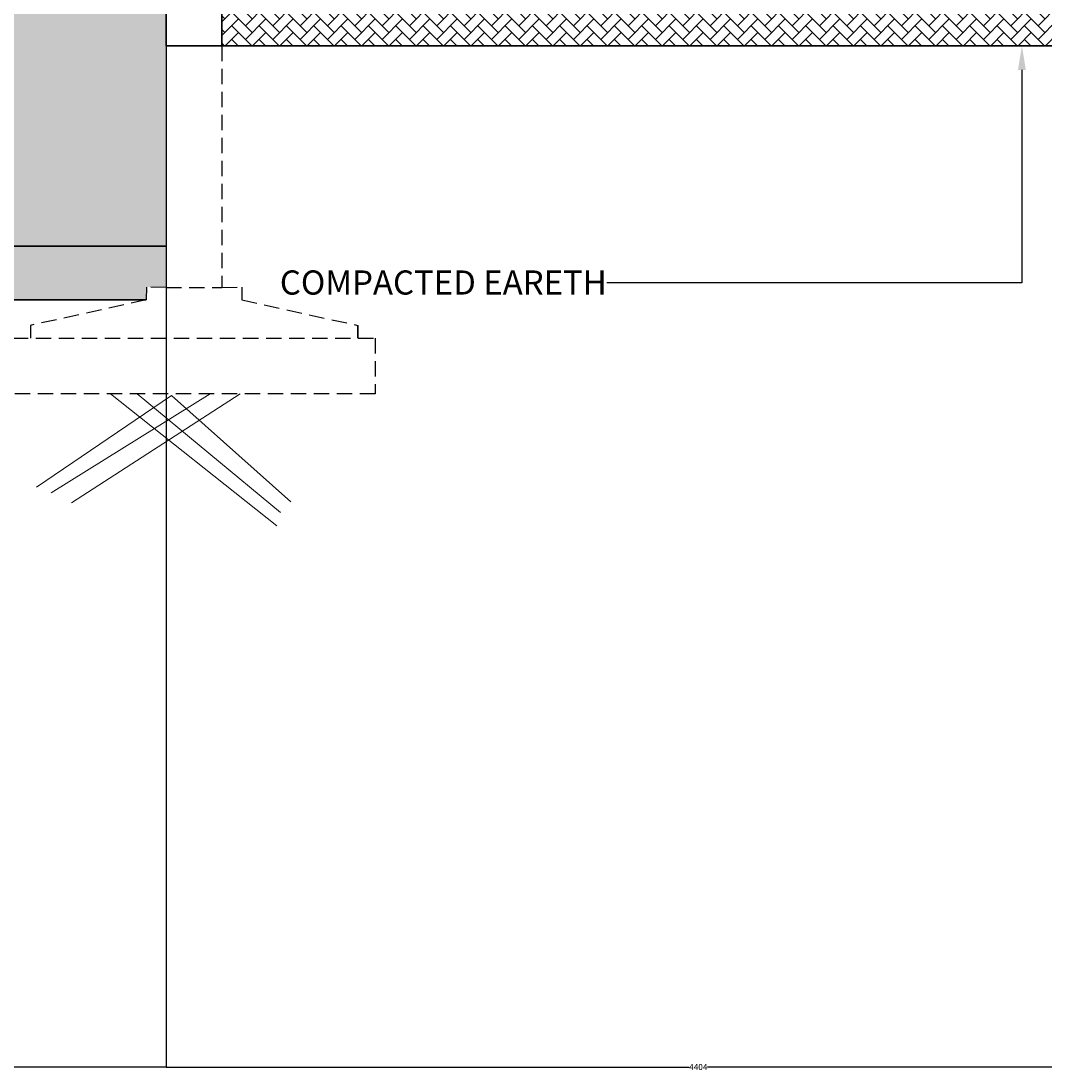
# Model space of a CAD drawing. Units: millimetres. Extents: x 1944 to 29915, y -10550 to 5909.
# Tile 10 of 24: x 11743 to 15981, y -10550 to -6203. Entities that reach past the tile are written whole.
import ezdxf
from ezdxf import colors
from ezdxf.entities.mleader import LeaderData, LeaderLine
from ezdxf.math import Vec2, Vec3

# ---------------------------------------------------------------- set-up
doc = ezdxf.new("R2010")
doc.units = ezdxf.units.MM
doc.header["$MEASUREMENT"] = 0
doc.linetypes.add('HIDDEN', pattern=[9.525, 6.35, -3.175])
for name, color, linetype, lineweight in [('A-ANNO-DIMS', 2, 'Continuous', 18), ('A-ANNO-TEXT', 7, 'Continuous', 25), ('A-FLOR-PATT', 252, 'Continuous', 13), ('A-SECT', 7, 'Continuous', 35), ('C-TOPO', 94, 'Continuous', 18), ('S-FNDN-HIDN', 1, 'HIDDEN', 25)]:
    doc.layers.add(name, color=color, linetype=linetype, lineweight=lineweight)
doc.styles.get("Standard").update_dxf_attribs({"font": 'arial.ttf'})
doc.dimstyles.get("Standard").update_dxf_attribs({"dimtxt": 25, "dimasz": 0.18, "dimexe": 0.18, "dimexo": 0.0625, "dimgap": 0.09, "dimtad": 0, "dimtih": 1, "dimtoh": 1, "dimdec": 0, "dimzin": 0, "dimdsep": 46, "dimtxsty": 'Standard', "dimcen": 0.09, "dimadec": 0, "dimazin": 0, "dimtfac": 1, "dimtdec": 0, "dimtofl": 0, "dimtmove": 0, "dimatfit": 3, "dimfxl": 1, "dimtolj": 1, "dimtzin": 0, "dimarcsym": 0})

# ---------------------------------------------------------------- blocks, each defined once
blk = doc.blocks.new('EARTH-COMPACT-SYMB')
for q in [(0, 60.9), (1053, 0)]:
    blk.add_line((559.8, 441.1), q)
blk = doc.blocks.new('*D86')
at = {"layer": 'A-ANNO-DIMS', "color": 0, "lineweight": -2, "transparency": 16777216}
for p, q in [((12344, -6305.8), (12344, -10533.3)), ((6418.3, -6851), (6418.3, -10533.3)), ((6418.5, -10533.1), (9343.7, -10533.1)), ((12343.8, -10533.1), (9418.6, -10533.1))]:
    blk.add_line(p, q, dxfattribs=at)
at = {"layer": 'A-ANNO-DIMS', "color": 0, "transparency": 16777216}
for points in [[(6418.5, -10533.1), (6418.5, -10533.1), (6418.3, -10533.1)], [(12343.8, -10533.1), (12343.8, -10533.1), (12344, -10533.1)]]:
    blk.add_solid(points, dxfattribs=at)
at = {"layer": 'Defpoints', "color": 0, "transparency": 16777216}
for p in [(12344, -6305.8), (6418.3, -6851), (12344, -10533.1)]:
    blk.add_point(p, dxfattribs=at)
at = {"layer": 'A-ANNO-DIMS', "color": 0, "transparency": 16777216, "insert": (9381.1, -10533.1), "char_height": 25, "attachment_point": 5}
blk.add_mtext('\\A1;5926', dxfattribs=at)
blk = doc.blocks.new('*D87')
at = {"layer": 'A-ANNO-DIMS', "color": 0, "lineweight": -2, "transparency": 16777216}
for p, q in [((12344, -6305.8), (12344, -10533.3)), ((16747.8, -6305.8), (16747.8, -10533.3)), ((12344.2, -10533.1), (14508, -10533.1)), ((16747.6, -10533.1), (14583.8, -10533.1))]:
    blk.add_line(p, q, dxfattribs=at)
at = {"layer": 'A-ANNO-DIMS', "color": 0, "transparency": 16777216}
for points in [[(12344.2, -10533.1), (12344.2, -10533.1), (12344, -10533.1)], [(16747.6, -10533.1), (16747.6, -10533.1), (16747.8, -10533.1)]]:
    blk.add_solid(points, dxfattribs=at)
at = {"layer": 'Defpoints', "color": 0, "transparency": 16777216}
for p in [(12344, -6305.8), (16747.8, -6305.8), (16747.8, -10533.1)]:
    blk.add_point(p, dxfattribs=at)
at = {"layer": 'A-ANNO-DIMS', "color": 0, "transparency": 16777216, "insert": (14545.9, -10533.1), "char_height": 25, "attachment_point": 5}
blk.add_mtext('\\A1;4404', dxfattribs=at)

msp = doc.modelspace()

# ---------------------------------------------------------------- hatches: boundary and pattern name
at = {"layer": 'A-FLOR-PATT'}
h = msp.add_hatch(dxfattribs=at)
h.set_pattern_fill('AR-HBONE', color=256, scale=10)
h.paths.add_polyline_path([(12343.981, -6305.752), (12343.981, -6061.05), (11445.739, -6061.05), (11445.739, -6850.967), (11265.739, -6850.967), (10496.11, -6850.967), (10496.11, -6990.545), (6648.315, -6990.545), (6648.315, -7135.877), (12343.981, -7135.877)])
h = msp.add_hatch(dxfattribs=at)
h.set_pattern_fill('AR-HBONE', color=256, scale=10)
h.paths.add_polyline_path([(12573.981, -6073.852), (12573.981, -6305.752), (16747.828, -6305.752), (16747.828, -6073.852)])
h = msp.add_hatch(dxfattribs=at)
h.set_pattern_fill('AR-HBONE', color=256, scale=10)
h.paths.add_polyline_path([(12343.981, -7135.877), (6648.315, -7135.877), (6648.315, -7210.967), (6648.315, -7357.264), (12261.31, -7357.264), (12261.952, -7304.748), (12343.981, -7305.752)])

# ---------------------------------------------------------------- linework, layer by layer
at = {"layer": 'A-SECT'}
for p, q in [((12573.981, -6305.752), (16747.828, -6305.752)), ((6648.315, -7135.877), (12343.981, -7135.877)), ((12261.31, -7357.264), (6648.315, -7357.264)), ((13136.605, -7463.338), (13136.605, -7516.218))]:
    msp.add_line(p, q, dxfattribs=at)
msp.add_lwpolyline([(12343.981, -5945.752), (12573.981, -5945.752), (12573.981, -6305.752), (12343.981, -6305.752)], close=True, dxfattribs=at)
at = {"layer": 'C-TOPO'}
for p, q in [((12525.518, -7746.218), (11867.22, -8155.847)), ((12650.473, -7746.218), (11951.031, -8196.963)), ((12112.558, -7746.218), (12801.333, -8292.9)), ((12223.798, -7746.218), (12816.571, -8238.079))]:
    msp.add_line(p, q, dxfattribs=at)
at = {"layer": 'S-FNDN-HIDN', "ltscale": 10}
for p, q in [((12343.981, -6305.752), (12343.981, -7305.752)), ((12573.981, -6305.752), (12573.981, -7305.752)), ((12261.952, -7304.748), (12261.31, -7357.264)), ((12343.981, -7305.752), (12261.952, -7304.748)), ((12343.981, -7305.752), (12573.981, -7305.752)), ((12573.981, -7305.752), (12656.01, -7304.748)), ((12656.01, -7304.748), (12656.652, -7357.264)), ((12261.31, -7357.264), (11781.357, -7463.338)), ((12656.652, -7357.264), (13136.605, -7463.338)), ((11781.357, -7463.338), (11781.357, -7516.218))]:
    msp.add_line(p, q, dxfattribs=at)
msp.add_lwpolyline([(11708.981, -7516.218), (13208.981, -7516.218), (13208.981, -7746.218), (11708.981, -7746.218)], close=True, dxfattribs=at)

# ---------------------------------------------------------------- block references
at = {"layer": 'C-TOPO'}
msp.add_blockref('EARTH-COMPACT-SYMB', (11806.267, -8193.917), dxfattribs=at)

# ---------------------------------------------------------------- dimensions: what is measured, and where the dimension line sits
at = {"layer": 'A-ANNO-DIMS'}
for base, p1, p2, picture, middle in [((12343.981, -10533.115), (6418.315, -6850.967), (12343.981, -6305.752), '*D86', (9381.148, -10533.115)), ((16747.828, -10533.115), (12343.981, -6305.752), (16747.828, -6305.752), '*D87', (14545.905, -10533.115))]:
    dim = msp.add_linear_dim(base=base, p1=p1, p2=p2, dimstyle='Standard', override={"dimdec": 0, "dimlfac": 1, "dimrnd": 0, "dimzin": 0, "dimdsep": 46, "dimlunit": 2}, dxfattribs=at)
    dim.commit()
    dim.dimension.update_dxf_attribs({"geometry": picture, "text_midpoint": middle})

# ---------------------------------------------------------------- leaders
at = {"layer": 'A-ANNO-TEXT'}
ml = msp.add_multileader_mtext('Standard', dxfattribs=at)
ml.set_content('COMPACTED EARETH ', color=256)
ml.set_leader_properties()
ml.build(insert=Vec2(0, 0))
ml.multileader.update_dxf_attribs({"dogleg_length": 568.936, "arrow_head_size": 100})
ctx = ml.context
ctx.base_point, ctx.char_height, ctx.arrow_head_size, ctx.landing_gap_size, ctx.plane_origin = Vec3(12687.303, -7286.495), 100, 100, 0.09, Vec3(14736.227, -7286.495)
ctx.text_align_type = 2
notes = []
notes.append((ctx, [(0, (1, 1, 0), (14736.227, -7286.495), (-1, 0), 568.936, [(0, [(15885.282, -6305.752), (15885.282, -7286.495)], 0, [])])]))
ctx.mtext.insert, ctx.mtext.alignment, ctx.mtext.flow_direction = Vec3(14167.202, -7235.642), 3, 5
for ctx, leaders in notes:
    for number, flags, end, landing, length, lines in leaders:
        leader = LeaderData()
        leader.index, (leader.has_last_leader_line, leader.has_dogleg_vector, leader.attachment_direction) = number, flags
        leader.last_leader_point, leader.dogleg_vector, leader.dogleg_length = Vec3(end), Vec3(landing), length
        for number, points, colour, breaks in lines:
            line = LeaderLine()
            line.index, line.vertices, line.color, line.breaks = number, Vec3.list(points), colors.encode_raw_color(colour), breaks
            leader.lines.append(line)
        ctx.leaders.append(leader)

doc.saveas('drawing.dxf')
